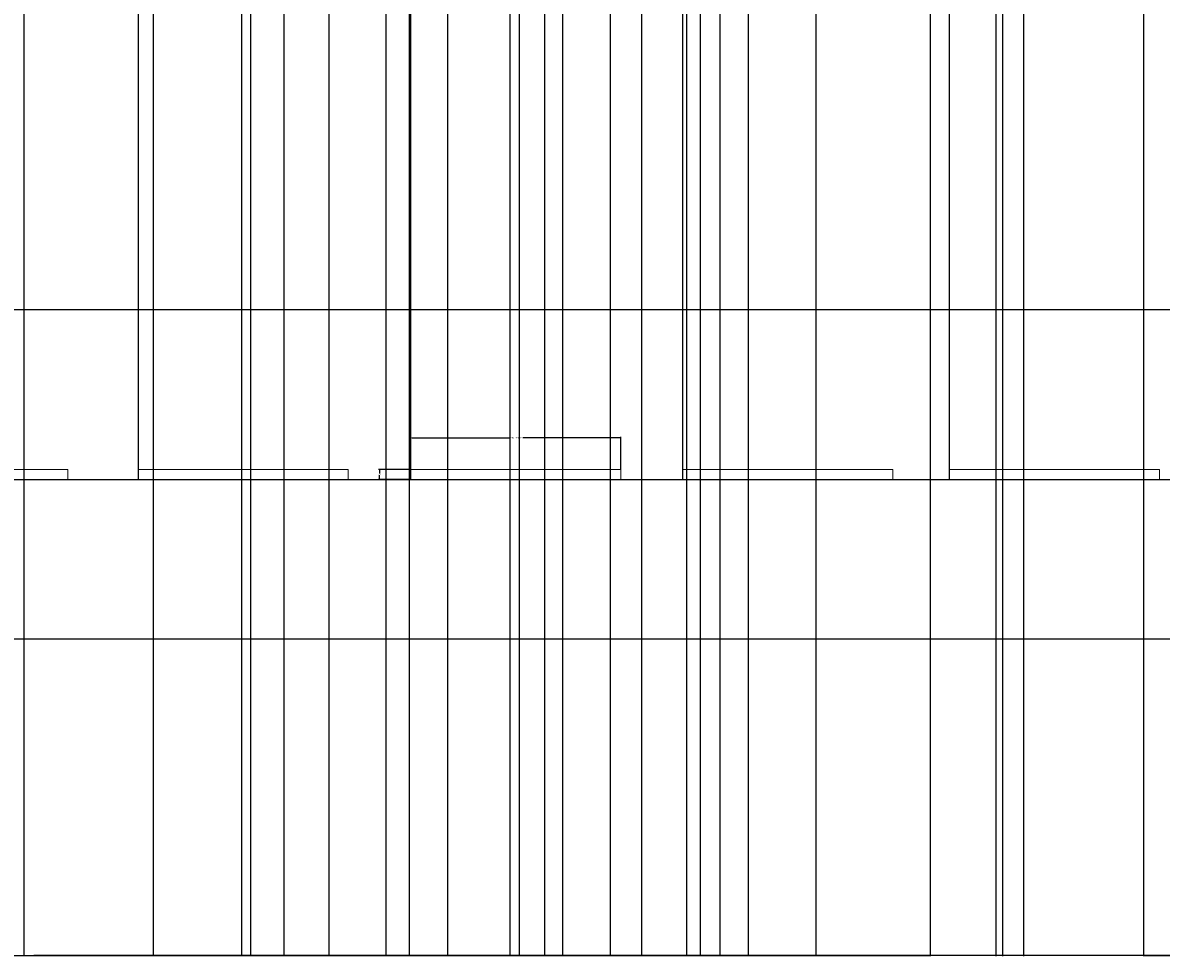
# Model space of a CAD drawing. Units: inches. Extents: x 818 to 1898, y 976 to 2364.
# Tile 14 of 96: x 1207 to 1434, y 976 to 1162. Entities that reach past the tile are written whole.
import ezdxf

# ---------------------------------------------------------------- set-up
doc = ezdxf.new("R2010")
doc.units = ezdxf.units.IN
doc.header["$LTSCALE"] = 5
doc.header["$MEASUREMENT"] = 0
for name, color, linetype, lineweight in [('A-ANNO-DIMS', 2, 'Continuous', 18), ('C-ROAD', 8, 'Continuous', 25), ('C-ROAD-MRKG', 7, 'Continuous', 13)]:
    doc.layers.add(name, color=color, linetype=linetype, lineweight=lineweight)
doc.styles.get("Standard").update_dxf_attribs({"font": 'arial.ttf'})
doc.dimstyles.get("Standard").update_dxf_attribs({"dimtxt": 0.18, "dimasz": 0.18, "dimexe": 0.18, "dimexo": 0.0625, "dimgap": 0.09, "dimtad": 0, "dimtih": 1, "dimtoh": 1, "dimdec": 4, "dimzin": 0, "dimdsep": 46, "dimtxsty": 'Standard', "dimcen": 0.09, "dimadec": 0, "dimazin": 0, "dimtfac": 1, "dimtdec": 4, "dimtofl": 0, "dimtmove": 0, "dimatfit": 3, "dimfxl": 1, "dimtolj": 1, "dimtzin": 0, "dimarcsym": 0})

# ---------------------------------------------------------------- blocks, each defined once
blk = doc.blocks.new('LANE-STRIPE')
at = {"ltscale": 5}
for p, q in [((0, 2), (42, 2)), ((0, 2), (0, 0)), ((0, 0), (42, 0)), ((42, 2), (42, 0))]:
    blk.add_line(p, q, dxfattribs=at)
blk = doc.blocks.new('*D32')
at = {"layer": 'A-ANNO-DIMS', "color": 0, "lineweight": -2, "ltscale": 5, "transparency": 16777216}
for p, q in [((1284.17, 1073.12), (1284.17, 1079.54)), ((1326.17, 1073.12), (1326.17, 1079.54)), ((1284.35, 1079.36), (1303.79, 1079.36)), ((1325.99, 1079.36), (1306.55, 1079.36))]:
    blk.add_line(p, q, dxfattribs=at)
at = {"layer": 'A-ANNO-DIMS', "color": 0, "ltscale": 5, "transparency": 16777216}
for points in [[(1284.35, 1079.39), (1284.35, 1079.33), (1284.17, 1079.36)], [(1325.99, 1079.39), (1325.99, 1079.33), (1326.17, 1079.36)]]:
    blk.add_solid(points, dxfattribs=at)
at = {"layer": 'Defpoints', "color": 0, "ltscale": 5, "transparency": 16777216}
for p in [(1284.17, 1079.36), (1284.17, 1073.06), (1326.17, 1073.06)]:
    blk.add_point(p, dxfattribs=at)
at = {"layer": 'A-ANNO-DIMS', "color": 0, "ltscale": 5, "transparency": 16777216, "insert": (1305.17, 1079.36), "char_height": 0.18, "attachment_point": 5}
blk.add_mtext('\\A1;LANE STRIPE 42 TYP.', dxfattribs=at)
blk = doc.blocks.new('*D33')
at = {"layer": 'A-ANNO-DIMS', "color": 0, "lineweight": -2, "ltscale": 5, "transparency": 16777216}
for p, q in [((1284.11, 1073.06), (1277.69, 1073.06)), ((1277.87, 1072.88), (1277.87, 1072.24)), ((1284.11, 1071.06), (1277.69, 1071.06)), ((1277.87, 1071.24), (1277.87, 1071.87))]:
    blk.add_line(p, q, dxfattribs=at)
at = {"layer": 'A-ANNO-DIMS', "color": 0, "ltscale": 5, "transparency": 16777216}
for points in [[(1277.84, 1072.88), (1277.9, 1072.88), (1277.87, 1073.06)], [(1277.84, 1071.24), (1277.9, 1071.24), (1277.87, 1071.06)]]:
    blk.add_solid(points, dxfattribs=at)
at = {"layer": 'Defpoints', "color": 0, "ltscale": 5, "transparency": 16777216}
for p in [(1284.17, 1073.06), (1277.87, 1071.06), (1284.17, 1071.06)]:
    blk.add_point(p, dxfattribs=at)
at = {"layer": 'A-ANNO-DIMS', "color": 0, "ltscale": 5, "transparency": 16777216, "insert": (1277.87, 1072.06), "char_height": 0.18, "attachment_point": 5}
blk.add_mtext('\\A1;2 TYP.', dxfattribs=at)
blk = doc.blocks.new('*D56')
at = {"layer": 'A-ANNO-DIMS', "color": 0, "lineweight": -2, "ltscale": 5, "transparency": 16777216}
for p, q in [((885.95, 1167.31), (885.95, 975.66)), ((1828.91, 1167.31), (1828.91, 975.66)), ((886.13, 975.84), (1357.14, 975.84)), ((1828.73, 975.84), (1357.72, 975.84))]:
    blk.add_line(p, q, dxfattribs=at)
at = {"layer": 'A-ANNO-DIMS', "color": 0, "ltscale": 5, "transparency": 16777216}
for points in [[(886.13, 975.87), (886.13, 975.81), (885.95, 975.84)], [(1828.73, 975.87), (1828.73, 975.81), (1828.91, 975.84)]]:
    blk.add_solid(points, dxfattribs=at)
at = {"layer": 'Defpoints', "color": 0, "ltscale": 5, "transparency": 16777216}
for p in [(885.95, 1167.37), (1828.91, 1167.37), (1828.91, 975.84)]:
    blk.add_point(p, dxfattribs=at)
at = {"layer": 'A-ANNO-DIMS', "color": 0, "ltscale": 5, "transparency": 16777216, "insert": (1357.43, 975.84), "char_height": 0.18, "attachment_point": 5}
blk.add_mtext('\\A1;943', dxfattribs=at)
blk = doc.blocks.new('*D58')
at = {"layer": 'A-ANNO-DIMS', "color": 0, "lineweight": -2, "ltscale": 5, "transparency": 16777216}
for p, q in [((881.51, 1159.31), (881.51, 975.66)), ((1834.44, 1145.13), (1834.44, 975.66)), ((881.69, 975.84), (1357.68, 975.84)), ((1834.26, 975.84), (1358.26, 975.84))]:
    blk.add_line(p, q, dxfattribs=at)
at = {"layer": 'A-ANNO-DIMS', "color": 0, "ltscale": 5, "transparency": 16777216}
for points in [[(881.69, 975.87), (881.69, 975.81), (881.51, 975.84)], [(1834.26, 975.87), (1834.26, 975.81), (1834.44, 975.84)]]:
    blk.add_solid(points, dxfattribs=at)
at = {"layer": 'Defpoints', "color": 0, "ltscale": 5, "transparency": 16777216}
for p in [(881.51, 1159.38), (1834.44, 1145.19), (1834.44, 975.84)]:
    blk.add_point(p, dxfattribs=at)
at = {"layer": 'A-ANNO-DIMS', "color": 0, "ltscale": 5, "transparency": 16777216, "insert": (1357.97, 975.84), "char_height": 0.18, "attachment_point": 5}
blk.add_mtext('\\A1;953', dxfattribs=at)
blk = doc.blocks.new('*D59')
at = {"layer": 'A-ANNO-DIMS', "color": 0, "lineweight": -2, "ltscale": 5, "transparency": 16777216}
for p, q in [((1251.64, 2300.39), (818.03, 2300.39)), ((818.21, 2300.21), (818.21, 1669.95)), ((818.21, 1039.32), (818.21, 1669.59)), ((896.05, 1039.14), (818.03, 1039.14))]:
    blk.add_line(p, q, dxfattribs=at)
at = {"layer": 'A-ANNO-DIMS', "color": 0, "ltscale": 5, "transparency": 16777216}
for points in [[(818.18, 2300.21), (818.24, 2300.21), (818.21, 2300.39)], [(818.18, 1039.32), (818.24, 1039.32), (818.21, 1039.14)]]:
    blk.add_solid(points, dxfattribs=at)
at = {"layer": 'Defpoints', "color": 0, "ltscale": 5, "transparency": 16777216}
for p in [(818.21, 2300.39), (1251.71, 2300.39), (896.11, 1039.14)]:
    blk.add_point(p, dxfattribs=at)
at = {"layer": 'A-ANNO-DIMS', "color": 0, "ltscale": 5, "transparency": 16777216, "insert": (818.21, 1669.77), "char_height": 0.18, "attachment_point": 5}
blk.add_mtext('\\A1;1261.2', dxfattribs=at)
blk = doc.blocks.new('*D62')
at = {"layer": 'A-ANNO-DIMS', "color": 0, "lineweight": -2, "ltscale": 5, "transparency": 16777216}
for p, q in [((1116.19, 1235.9), (1116.19, 975.66)), ((1406.73, 1235.9), (1406.73, 975.66)), ((1116.37, 975.84), (1260.99, 975.84)), ((1406.55, 975.84), (1261.92, 975.84))]:
    blk.add_line(p, q, dxfattribs=at)
at = {"layer": 'A-ANNO-DIMS', "color": 0, "ltscale": 5, "transparency": 16777216}
for points in [[(1116.37, 975.87), (1116.37, 975.81), (1116.19, 975.84)], [(1406.55, 975.87), (1406.55, 975.81), (1406.73, 975.84)]]:
    blk.add_solid(points, dxfattribs=at)
at = {"layer": 'Defpoints', "color": 0, "ltscale": 5, "transparency": 16777216}
for p in [(1116.19, 1235.96), (1406.73, 1235.96), (1406.73, 975.84)]:
    blk.add_point(p, dxfattribs=at)
at = {"layer": 'A-ANNO-DIMS', "color": 0, "ltscale": 5, "transparency": 16777216, "insert": (1261.46, 975.84), "char_height": 0.18, "attachment_point": 5}
blk.add_mtext('\\A1;290.54', dxfattribs=at)
blk = doc.blocks.new('*D65')
at = {"layer": 'A-ANNO-DIMS', "color": 0, "lineweight": -2, "ltscale": 5, "transparency": 16777216}
for p, q in [((1430.73, 1346.02), (1430.73, 975.66)), ((1714.73, 1346.02), (1714.73, 975.66)), ((1430.91, 975.84), (1572.44, 975.84)), ((1714.55, 975.84), (1573.02, 975.84))]:
    blk.add_line(p, q, dxfattribs=at)
at = {"layer": 'A-ANNO-DIMS', "color": 0, "ltscale": 5, "transparency": 16777216}
for points in [[(1430.91, 975.87), (1430.91, 975.81), (1430.73, 975.84)], [(1714.55, 975.87), (1714.55, 975.81), (1714.73, 975.84)]]:
    blk.add_solid(points, dxfattribs=at)
at = {"layer": 'Defpoints', "color": 0, "ltscale": 5, "transparency": 16777216}
for p in [(1430.73, 1346.08), (1714.73, 1346.08), (1714.73, 975.84)]:
    blk.add_point(p, dxfattribs=at)
at = {"layer": 'A-ANNO-DIMS', "color": 0, "ltscale": 5, "transparency": 16777216, "insert": (1572.73, 975.84), "char_height": 0.18, "attachment_point": 5}
blk.add_mtext('\\A1;284', dxfattribs=at)
blk = doc.blocks.new('*D89')
at = {"layer": 'A-ANNO-DIMS', "color": 0, "lineweight": -2, "ltscale": 5, "transparency": 16777216}
for p, q in [((905.01, 1071.06), (1897.92, 1071.06)), ((1897.74, 1070.88), (1897.74, 1055.28)), ((1897.74, 1039.32), (1897.74, 1054.92)), ((896.18, 1039.14), (1897.92, 1039.14))]:
    blk.add_line(p, q, dxfattribs=at)
at = {"layer": 'A-ANNO-DIMS', "color": 0, "ltscale": 5, "transparency": 16777216}
for points in [[(1897.71, 1070.88), (1897.77, 1070.88), (1897.74, 1071.06)], [(1897.71, 1039.32), (1897.77, 1039.32), (1897.74, 1039.14)]]:
    blk.add_solid(points, dxfattribs=at)
at = {"layer": 'Defpoints', "color": 0, "ltscale": 5, "transparency": 16777216}
for p in [(904.95, 1071.06), (1897.74, 1071.06), (896.11, 1039.14)]:
    blk.add_point(p, dxfattribs=at)
at = {"layer": 'A-ANNO-DIMS', "color": 0, "ltscale": 5, "transparency": 16777216, "insert": (1897.74, 1055.1), "char_height": 0.18, "attachment_point": 5}
blk.add_mtext('\\A1;31.91', dxfattribs=at)
blk = doc.blocks.new('*D95')
at = {"layer": 'A-ANNO-DIMS', "color": 0, "lineweight": -2, "ltscale": 5, "transparency": 16777216}
for p, q in [((1173.54, 1071.12), (1173.54, 2363.87)), ((1229.65, 1071.12), (1229.65, 2363.87)), ((1173.72, 2363.69), (1201.29, 2363.69)), ((1229.47, 2363.69), (1201.9, 2363.69))]:
    blk.add_line(p, q, dxfattribs=at)
at = {"layer": 'A-ANNO-DIMS', "color": 0, "ltscale": 5, "transparency": 16777216}
for points in [[(1173.72, 2363.72), (1173.72, 2363.66), (1173.54, 2363.69)], [(1229.47, 2363.72), (1229.47, 2363.66), (1229.65, 2363.69)]]:
    blk.add_solid(points, dxfattribs=at)
at = {"layer": 'Defpoints', "color": 0, "ltscale": 5, "transparency": 16777216}
for p in [(1229.65, 2363.69), (1173.54, 1071.06), (1229.65, 1071.06)]:
    blk.add_point(p, dxfattribs=at)
at = {"layer": 'A-ANNO-DIMS', "color": 0, "ltscale": 5, "transparency": 16777216, "insert": (1201.59, 2363.69), "char_height": 0.18, "attachment_point": 5}
blk.add_mtext('\\A1;56.1', dxfattribs=at)
blk = doc.blocks.new('*D96')
at = {"layer": 'A-ANNO-DIMS', "color": 0, "lineweight": -2, "ltscale": 5, "transparency": 16777216}
for p, q in [((1229.65, 1071.12), (1229.65, 2363.87)), ((1284.17, 1071.12), (1284.17, 2363.87)), ((1229.83, 2363.69), (1256.52, 2363.69)), ((1283.99, 2363.69), (1257.3, 2363.69))]:
    blk.add_line(p, q, dxfattribs=at)
at = {"layer": 'A-ANNO-DIMS', "color": 0, "ltscale": 5, "transparency": 16777216}
for points in [[(1229.83, 2363.72), (1229.83, 2363.66), (1229.65, 2363.69)], [(1283.99, 2363.72), (1283.99, 2363.66), (1284.17, 2363.69)]]:
    blk.add_solid(points, dxfattribs=at)
at = {"layer": 'Defpoints', "color": 0, "ltscale": 5, "transparency": 16777216}
for p in [(1284.17, 2363.69), (1229.65, 1071.06), (1284.17, 1071.06)]:
    blk.add_point(p, dxfattribs=at)
at = {"layer": 'A-ANNO-DIMS', "color": 0, "ltscale": 5, "transparency": 16777216, "insert": (1256.91, 2363.69), "char_height": 0.18, "attachment_point": 5}
blk.add_mtext('\\A1;54.52', dxfattribs=at)
blk = doc.blocks.new('*D97')
at = {"layer": 'A-ANNO-DIMS', "color": 0, "lineweight": -2, "ltscale": 5, "transparency": 16777216}
for p, q in [((1284.17, 1071.12), (1284.17, 2363.87)), ((1338.54, 1071.12), (1338.54, 2363.87)), ((1284.35, 2363.69), (1310.96, 2363.69)), ((1338.36, 2363.69), (1311.75, 2363.69))]:
    blk.add_line(p, q, dxfattribs=at)
at = {"layer": 'A-ANNO-DIMS', "color": 0, "ltscale": 5, "transparency": 16777216}
for points in [[(1284.35, 2363.72), (1284.35, 2363.66), (1284.17, 2363.69)], [(1338.36, 2363.72), (1338.36, 2363.66), (1338.54, 2363.69)]]:
    blk.add_solid(points, dxfattribs=at)
at = {"layer": 'Defpoints', "color": 0, "ltscale": 5, "transparency": 16777216}
for p in [(1338.54, 2363.69), (1284.17, 1071.06), (1338.54, 1071.06)]:
    blk.add_point(p, dxfattribs=at)
at = {"layer": 'A-ANNO-DIMS', "color": 0, "ltscale": 5, "transparency": 16777216, "insert": (1311.36, 2363.69), "char_height": 0.18, "attachment_point": 5}
blk.add_mtext('\\A1;54.37', dxfattribs=at)
blk = doc.blocks.new('*D98')
at = {"layer": 'A-ANNO-DIMS', "color": 0, "lineweight": -2, "ltscale": 5, "transparency": 16777216}
for p, q in [((1338.54, 1071.12), (1338.54, 2363.87)), ((1391.88, 1071.12), (1391.88, 2363.87)), ((1338.72, 2363.69), (1364.81, 2363.69)), ((1391.7, 2363.69), (1365.6, 2363.69))]:
    blk.add_line(p, q, dxfattribs=at)
at = {"layer": 'A-ANNO-DIMS', "color": 0, "ltscale": 5, "transparency": 16777216}
for points in [[(1338.72, 2363.72), (1338.72, 2363.66), (1338.54, 2363.69)], [(1391.7, 2363.72), (1391.7, 2363.66), (1391.88, 2363.69)]]:
    blk.add_solid(points, dxfattribs=at)
at = {"layer": 'Defpoints', "color": 0, "ltscale": 5, "transparency": 16777216}
for p in [(1391.88, 2363.69), (1338.54, 1071.06), (1391.88, 1071.06)]:
    blk.add_point(p, dxfattribs=at)
at = {"layer": 'A-ANNO-DIMS', "color": 0, "ltscale": 5, "transparency": 16777216, "insert": (1365.21, 2363.69), "char_height": 0.18, "attachment_point": 5}
blk.add_mtext('\\A1;53.33', dxfattribs=at)
blk = doc.blocks.new('*D99')
at = {"layer": 'A-ANNO-DIMS', "color": 0, "lineweight": -2, "ltscale": 5, "transparency": 16777216}
for p, q in [((1391.88, 1071.12), (1391.88, 2363.87)), ((1449.82, 1071.12), (1449.82, 2363.87)), ((1392.06, 2363.69), (1420.45, 2363.69)), ((1449.64, 2363.69), (1421.24, 2363.69))]:
    blk.add_line(p, q, dxfattribs=at)
at = {"layer": 'A-ANNO-DIMS', "color": 0, "ltscale": 5, "transparency": 16777216}
for points in [[(1392.06, 2363.72), (1392.06, 2363.66), (1391.88, 2363.69)], [(1449.64, 2363.72), (1449.64, 2363.66), (1449.82, 2363.69)]]:
    blk.add_solid(points, dxfattribs=at)
at = {"layer": 'Defpoints', "color": 0, "ltscale": 5, "transparency": 16777216}
for p in [(1449.82, 2363.69), (1391.88, 1071.06), (1449.82, 1071.06)]:
    blk.add_point(p, dxfattribs=at)
at = {"layer": 'A-ANNO-DIMS', "color": 0, "ltscale": 5, "transparency": 16777216, "insert": (1420.85, 2363.69), "char_height": 0.18, "attachment_point": 5}
blk.add_mtext('\\A1;57.94', dxfattribs=at)
blk = doc.blocks.new('*D106')
at = {"layer": 'A-ANNO-DIMS', "color": 0, "lineweight": -2, "ltscale": 5, "transparency": 16777216}
for p, q in [((1164.56, 1248.4), (1164.56, 975.66)), ((1252.11, 1248.4), (1252.11, 975.66)), ((1164.74, 975.84), (1207.94, 975.84)), ((1251.93, 975.84), (1208.73, 975.84))]:
    blk.add_line(p, q, dxfattribs=at)
at = {"layer": 'A-ANNO-DIMS', "color": 0, "ltscale": 5, "transparency": 16777216}
for points in [[(1164.74, 975.87), (1164.74, 975.81), (1164.56, 975.84)], [(1251.93, 975.87), (1251.93, 975.81), (1252.11, 975.84)]]:
    blk.add_solid(points, dxfattribs=at)
at = {"layer": 'Defpoints', "color": 0, "ltscale": 5, "transparency": 16777216}
for p in [(1164.56, 1248.46), (1252.11, 1248.46), (1252.11, 975.84)]:
    blk.add_point(p, dxfattribs=at)
at = {"layer": 'A-ANNO-DIMS', "color": 0, "ltscale": 5, "transparency": 16777216, "insert": (1208.33, 975.84), "char_height": 0.18, "attachment_point": 5}
blk.add_mtext('\\A1;87.55', dxfattribs=at)
blk = doc.blocks.new('*D107')
at = {"layer": 'A-ANNO-DIMS', "color": 0, "lineweight": -2, "ltscale": 5, "transparency": 16777216}
for p, q in [((1339.32, 1250.56), (1339.32, 975.66)), ((1252.11, 1248.4), (1252.11, 975.66)), ((1252.29, 975.84), (1295.39, 975.84)), ((1339.14, 975.84), (1296.04, 975.84))]:
    blk.add_line(p, q, dxfattribs=at)
at = {"layer": 'A-ANNO-DIMS', "color": 0, "ltscale": 5, "transparency": 16777216}
for points in [[(1252.29, 975.87), (1252.29, 975.81), (1252.11, 975.84)], [(1339.14, 975.87), (1339.14, 975.81), (1339.32, 975.84)]]:
    blk.add_solid(points, dxfattribs=at)
at = {"layer": 'Defpoints', "color": 0, "ltscale": 5, "transparency": 16777216}
for p in [(1339.32, 1250.62), (1252.11, 1248.46), (1339.32, 975.84)]:
    blk.add_point(p, dxfattribs=at)
at = {"layer": 'A-ANNO-DIMS', "color": 0, "ltscale": 5, "transparency": 16777216, "insert": (1295.71, 975.84), "char_height": 0.18, "attachment_point": 5}
blk.add_mtext('\\A1;87.2', dxfattribs=at)
blk = doc.blocks.new('*D145')
at = {"layer": 'A-ANNO-DIMS', "color": 0, "lineweight": -2, "ltscale": 5, "transparency": 16777216}
for p, q in [((1197.39, 2122.31), (1197.39, 975.66)), ((1232.61, 2122.31), (1232.61, 975.66)), ((1197.57, 975.84), (1214.61, 975.84)), ((1232.43, 975.84), (1215.39, 975.84))]:
    blk.add_line(p, q, dxfattribs=at)
at = {"layer": 'A-ANNO-DIMS', "color": 0, "ltscale": 5, "transparency": 16777216}
for points in [[(1197.57, 975.87), (1197.57, 975.81), (1197.39, 975.84)], [(1232.43, 975.87), (1232.43, 975.81), (1232.61, 975.84)]]:
    blk.add_solid(points, dxfattribs=at)
at = {"layer": 'Defpoints', "color": 0, "ltscale": 5, "transparency": 16777216}
for p in [(1197.39, 2122.38), (1232.61, 2122.38), (1232.61, 975.84)]:
    blk.add_point(p, dxfattribs=at)
at = {"layer": 'A-ANNO-DIMS', "color": 0, "ltscale": 5, "transparency": 16777216, "insert": (1215, 975.84), "char_height": 0.18, "attachment_point": 5}
blk.add_mtext('\\A1;35.22', dxfattribs=at)
blk = doc.blocks.new('*D159')
at = {"layer": 'A-ANNO-DIMS', "color": 0, "lineweight": -2, "ltscale": 5, "transparency": 16777216}
for p, q in [((1206.73, 1687.02), (1206.73, 975.66)), ((1463.73, 1687.02), (1463.73, 975.66)), ((1206.91, 975.84), (1334.93, 975.84)), ((1463.55, 975.84), (1335.52, 975.84))]:
    blk.add_line(p, q, dxfattribs=at)
at = {"layer": 'A-ANNO-DIMS', "color": 0, "ltscale": 5, "transparency": 16777216}
for points in [[(1206.91, 975.87), (1206.91, 975.81), (1206.73, 975.84)], [(1463.55, 975.87), (1463.55, 975.81), (1463.73, 975.84)]]:
    blk.add_solid(points, dxfattribs=at)
at = {"layer": 'Defpoints', "color": 0, "ltscale": 5, "transparency": 16777216}
for p in [(1206.73, 1687.08), (1463.73, 1687.08), (1463.73, 975.84)]:
    blk.add_point(p, dxfattribs=at)
at = {"layer": 'A-ANNO-DIMS', "color": 0, "ltscale": 5, "transparency": 16777216, "insert": (1335.23, 975.84), "char_height": 0.18, "attachment_point": 5}
blk.add_mtext('\\A1;257', dxfattribs=at)
blk = doc.blocks.new('*D163')
at = {"layer": 'A-ANNO-DIMS', "color": 0, "lineweight": -2, "ltscale": 5, "transparency": 16777216}
for p, q in [((1365.15, 1501.02), (1365.15, 975.66)), ((1401.15, 1501.02), (1401.15, 975.66)), ((1365.33, 975.84), (1382.93, 975.84)), ((1400.97, 975.84), (1383.37, 975.84))]:
    blk.add_line(p, q, dxfattribs=at)
at = {"layer": 'A-ANNO-DIMS', "color": 0, "ltscale": 5, "transparency": 16777216}
for points in [[(1365.33, 975.87), (1365.33, 975.81), (1365.15, 975.84)], [(1400.97, 975.87), (1400.97, 975.81), (1401.15, 975.84)]]:
    blk.add_solid(points, dxfattribs=at)
at = {"layer": 'Defpoints', "color": 0, "ltscale": 5, "transparency": 16777216}
for p in [(1365.15, 1501.08), (1401.15, 1501.08), (1401.15, 975.84)]:
    blk.add_point(p, dxfattribs=at)
at = {"layer": 'A-ANNO-DIMS', "color": 0, "ltscale": 5, "transparency": 16777216, "insert": (1383.15, 975.84), "char_height": 0.18, "attachment_point": 5}
blk.add_mtext('\\A1;36', dxfattribs=at)
blk = doc.blocks.new('*D164')
at = {"layer": 'A-ANNO-DIMS', "color": 0, "lineweight": -2, "ltscale": 5, "transparency": 16777216}
for p, q in [((1206.73, 1501.02), (1206.73, 975.66)), ((1283.82, 1501.02), (1283.82, 975.66)), ((1206.91, 975.84), (1244.97, 975.84)), ((1283.64, 975.84), (1245.58, 975.84))]:
    blk.add_line(p, q, dxfattribs=at)
at = {"layer": 'A-ANNO-DIMS', "color": 0, "ltscale": 5, "transparency": 16777216}
for points in [[(1206.91, 975.87), (1206.91, 975.81), (1206.73, 975.84)], [(1283.64, 975.87), (1283.64, 975.81), (1283.82, 975.84)]]:
    blk.add_solid(points, dxfattribs=at)
at = {"layer": 'Defpoints', "color": 0, "ltscale": 5, "transparency": 16777216}
for p in [(1206.73, 1501.08), (1283.82, 1501.08), (1283.82, 975.84)]:
    blk.add_point(p, dxfattribs=at)
at = {"layer": 'A-ANNO-DIMS', "color": 0, "ltscale": 5, "transparency": 16777216, "insert": (1245.27, 975.84), "char_height": 0.18, "attachment_point": 5}
blk.add_mtext('\\A1;77.1', dxfattribs=at)
blk = doc.blocks.new('*D167')
at = {"layer": 'A-ANNO-DIMS', "color": 0, "lineweight": -2, "ltscale": 5, "transparency": 16777216}
for p, q in [((1345.97, 1486.18), (1345.97, 975.66)), ((1430.73, 1486.18), (1430.73, 975.66)), ((1346.15, 975.84), (1387.95, 975.84)), ((1430.55, 975.84), (1388.74, 975.84))]:
    blk.add_line(p, q, dxfattribs=at)
at = {"layer": 'A-ANNO-DIMS', "color": 0, "ltscale": 5, "transparency": 16777216}
for points in [[(1346.15, 975.87), (1346.15, 975.81), (1345.97, 975.84)], [(1430.55, 975.87), (1430.55, 975.81), (1430.73, 975.84)]]:
    blk.add_solid(points, dxfattribs=at)
at = {"layer": 'Defpoints', "color": 0, "ltscale": 5, "transparency": 16777216}
for p in [(1345.97, 1486.24), (1430.73, 1486.24), (1430.73, 975.84)]:
    blk.add_point(p, dxfattribs=at)
at = {"layer": 'A-ANNO-DIMS', "color": 0, "ltscale": 5, "transparency": 16777216, "insert": (1388.35, 975.84), "char_height": 0.18, "attachment_point": 5}
blk.add_mtext('\\A1;84.76', dxfattribs=at)
blk = doc.blocks.new('*D189')
at = {"layer": 'A-ANNO-DIMS', "color": 0, "lineweight": -2, "ltscale": 5, "transparency": 16777216}
for p, q in [((1430.73, 1346.02), (1430.73, 975.66)), ((1490.92, 1346.02), (1490.92, 975.66)), ((1430.91, 975.84), (1460.43, 975.84)), ((1490.74, 975.84), (1461.22, 975.84))]:
    blk.add_line(p, q, dxfattribs=at)
at = {"layer": 'A-ANNO-DIMS', "color": 0, "ltscale": 5, "transparency": 16777216}
for points in [[(1430.91, 975.87), (1430.91, 975.81), (1430.73, 975.84)], [(1490.74, 975.87), (1490.74, 975.81), (1490.92, 975.84)]]:
    blk.add_solid(points, dxfattribs=at)
at = {"layer": 'Defpoints', "color": 0, "ltscale": 5, "transparency": 16777216}
for p in [(1430.73, 1346.08), (1490.92, 1346.08), (1490.92, 975.84)]:
    blk.add_point(p, dxfattribs=at)
at = {"layer": 'A-ANNO-DIMS', "color": 0, "ltscale": 5, "transparency": 16777216, "insert": (1460.82, 975.84), "char_height": 0.18, "attachment_point": 5}
blk.add_mtext('\\A1;60.19', dxfattribs=at)
blk = doc.blocks.new('*D198')
at = {"layer": 'A-ANNO-DIMS', "color": 0, "lineweight": -2, "ltscale": 5, "transparency": 16777216}
for p, q in [((1741.84, 1545.02), (1741.84, 975.66)), ((1430.73, 1346.02), (1430.73, 975.66)), ((1430.91, 975.84), (1585.91, 975.84)), ((1741.66, 975.84), (1586.66, 975.84))]:
    blk.add_line(p, q, dxfattribs=at)
at = {"layer": 'A-ANNO-DIMS', "color": 0, "ltscale": 5, "transparency": 16777216}
for points in [[(1430.91, 975.87), (1430.91, 975.81), (1430.73, 975.84)], [(1741.66, 975.87), (1741.66, 975.81), (1741.84, 975.84)]]:
    blk.add_solid(points, dxfattribs=at)
at = {"layer": 'Defpoints', "color": 0, "ltscale": 5, "transparency": 16777216}
for p in [(1741.84, 1545.08), (1430.73, 1346.08), (1741.84, 975.84)]:
    blk.add_point(p, dxfattribs=at)
at = {"layer": 'A-ANNO-DIMS', "color": 0, "ltscale": 5, "transparency": 16777216, "insert": (1586.28, 975.84), "char_height": 0.18, "attachment_point": 5}
blk.add_mtext('\\A1;311.1', dxfattribs=at)
blk = doc.blocks.new('*D231')
at = {"layer": 'A-ANNO-DIMS', "color": 0, "lineweight": -2, "ltscale": 5, "transparency": 16777216}
for p, q in [((1303.93, 1952.98), (1303.93, 975.66)), ((1402.52, 1952.98), (1402.52, 975.66)), ((1304.11, 975.84), (1352.83, 975.84)), ((1402.34, 975.84), (1353.62, 975.84))]:
    blk.add_line(p, q, dxfattribs=at)
at = {"layer": 'A-ANNO-DIMS', "color": 0, "ltscale": 5, "transparency": 16777216}
for points in [[(1304.11, 975.87), (1304.11, 975.81), (1303.93, 975.84)], [(1402.34, 975.87), (1402.34, 975.81), (1402.52, 975.84)]]:
    blk.add_solid(points, dxfattribs=at)
at = {"layer": 'Defpoints', "color": 0, "ltscale": 5, "transparency": 16777216}
for p in [(1303.93, 1953.04), (1402.52, 1953.04), (1402.52, 975.84)]:
    blk.add_point(p, dxfattribs=at)
at = {"layer": 'A-ANNO-DIMS', "color": 0, "ltscale": 5, "transparency": 16777216, "insert": (1353.22, 975.84), "char_height": 0.18, "attachment_point": 5}
blk.add_mtext('\\A1;98.59', dxfattribs=at)
blk = doc.blocks.new('*D233')
at = {"layer": 'A-ANNO-DIMS', "color": 0, "lineweight": -2, "ltscale": 5, "transparency": 16777216}
for p, q in [((1267.73, 2044.02), (1267.73, 975.66)), ((1303.93, 2008.33), (1303.93, 975.66)), ((1267.91, 975.84), (1285.36, 975.84)), ((1303.75, 975.84), (1286.29, 975.84))]:
    blk.add_line(p, q, dxfattribs=at)
at = {"layer": 'A-ANNO-DIMS', "color": 0, "ltscale": 5, "transparency": 16777216}
for points in [[(1267.91, 975.87), (1267.91, 975.81), (1267.73, 975.84)], [(1303.75, 975.87), (1303.75, 975.81), (1303.93, 975.84)]]:
    blk.add_solid(points, dxfattribs=at)
at = {"layer": 'Defpoints', "color": 0, "ltscale": 5, "transparency": 16777216}
for p in [(1267.73, 2044.08), (1303.93, 2008.39), (1303.93, 975.84)]:
    blk.add_point(p, dxfattribs=at)
at = {"layer": 'A-ANNO-DIMS', "color": 0, "ltscale": 5, "transparency": 16777216, "insert": (1285.83, 975.84), "char_height": 0.18, "attachment_point": 5}
blk.add_mtext('\\A1;36.206', dxfattribs=at)
blk = doc.blocks.new('*D236')
at = {"layer": 'A-ANNO-DIMS', "color": 0, "lineweight": -2, "ltscale": 5, "transparency": 16777216}
for p, q in [((1310.91, 2026.14), (1310.91, 975.66)), ((1342.04, 2026.14), (1342.04, 975.66)), ((1311.09, 975.84), (1326.08, 975.84)), ((1341.86, 975.84), (1326.87, 975.84))]:
    blk.add_line(p, q, dxfattribs=at)
at = {"layer": 'A-ANNO-DIMS', "color": 0, "ltscale": 5, "transparency": 16777216}
for points in [[(1311.09, 975.87), (1311.09, 975.81), (1310.91, 975.84)], [(1341.86, 975.87), (1341.86, 975.81), (1342.04, 975.84)]]:
    blk.add_solid(points, dxfattribs=at)
at = {"layer": 'Defpoints', "color": 0, "ltscale": 5, "transparency": 16777216}
for p in [(1310.91, 2026.21), (1342.04, 2026.21), (1342.04, 975.84)]:
    blk.add_point(p, dxfattribs=at)
at = {"layer": 'A-ANNO-DIMS', "color": 0, "ltscale": 5, "transparency": 16777216, "insert": (1326.48, 975.84), "char_height": 0.18, "attachment_point": 5}
blk.add_mtext('\\A1;31.14', dxfattribs=at)
blk = doc.blocks.new('*D245')
at = {"layer": 'A-ANNO-DIMS', "color": 0, "lineweight": -2, "ltscale": 5, "transparency": 16777216}
for p, q in [((1291.48, 1599.31), (1291.48, 975.66)), ((1314.49, 1599.31), (1314.49, 975.66)), ((1291.66, 975.84), (1302.61, 975.84)), ((1314.31, 975.84), (1303.36, 975.84))]:
    blk.add_line(p, q, dxfattribs=at)
at = {"layer": 'A-ANNO-DIMS', "color": 0, "ltscale": 5, "transparency": 16777216}
for points in [[(1291.66, 975.87), (1291.66, 975.81), (1291.48, 975.84)], [(1314.31, 975.87), (1314.31, 975.81), (1314.49, 975.84)]]:
    blk.add_solid(points, dxfattribs=at)
at = {"layer": 'Defpoints', "color": 0, "ltscale": 5, "transparency": 16777216}
for p in [(1291.48, 1599.37), (1314.49, 1599.37), (1314.49, 975.84)]:
    blk.add_point(p, dxfattribs=at)
at = {"layer": 'A-ANNO-DIMS', "color": 0, "ltscale": 5, "transparency": 16777216, "insert": (1302.98, 975.84), "char_height": 0.18, "attachment_point": 5}
blk.add_mtext('\\A1;23.01', dxfattribs=at)
blk = doc.blocks.new('*D251')
at = {"layer": 'A-ANNO-DIMS', "color": 0, "lineweight": -2, "ltscale": 5, "transparency": 16777216}
for p, q in [((1250.3, 1878.33), (1250.3, 975.66)), ((1258.73, 1878.33), (1258.73, 975.66)), ((1250.48, 975.84), (1254.12, 975.84)), ((1258.55, 975.84), (1254.91, 975.84))]:
    blk.add_line(p, q, dxfattribs=at)
at = {"layer": 'A-ANNO-DIMS', "color": 0, "ltscale": 5, "transparency": 16777216}
for points in [[(1250.48, 975.87), (1250.48, 975.81), (1250.3, 975.84)], [(1258.55, 975.87), (1258.55, 975.81), (1258.73, 975.84)]]:
    blk.add_solid(points, dxfattribs=at)
at = {"layer": 'Defpoints', "color": 0, "ltscale": 5, "transparency": 16777216}
for p in [(1250.3, 1878.39), (1258.73, 1878.39), (1258.73, 975.84)]:
    blk.add_point(p, dxfattribs=at)
at = {"layer": 'A-ANNO-DIMS', "color": 0, "ltscale": 5, "transparency": 16777216, "insert": (1254.51, 975.84), "char_height": 0.18, "attachment_point": 5}
blk.add_mtext('\\A1;8.422', dxfattribs=at)
blk = doc.blocks.new('*D252')
at = {"layer": 'A-ANNO-DIMS', "color": 0, "lineweight": -2, "ltscale": 5, "transparency": 16777216}
for p, q in [((1330.3, 2053.02), (1330.3, 975.66)), ((1388.03, 2053.02), (1388.03, 975.66)), ((1330.48, 975.84), (1358.77, 975.84)), ((1387.85, 975.84), (1359.56, 975.84))]:
    blk.add_line(p, q, dxfattribs=at)
at = {"layer": 'A-ANNO-DIMS', "color": 0, "ltscale": 5, "transparency": 16777216}
for points in [[(1330.48, 975.87), (1330.48, 975.81), (1330.3, 975.84)], [(1387.85, 975.87), (1387.85, 975.81), (1388.03, 975.84)]]:
    blk.add_solid(points, dxfattribs=at)
at = {"layer": 'Defpoints', "color": 0, "ltscale": 5, "transparency": 16777216}
for p in [(1330.3, 2053.08), (1388.03, 2053.08), (1388.03, 975.84)]:
    blk.add_point(p, dxfattribs=at)
at = {"layer": 'A-ANNO-DIMS', "color": 0, "ltscale": 5, "transparency": 16777216, "insert": (1359.17, 975.84), "char_height": 0.18, "attachment_point": 5}
blk.add_mtext('\\A1;57.73', dxfattribs=at)
blk = doc.blocks.new('*D254')
at = {"layer": 'A-ANNO-DIMS', "color": 0, "lineweight": -2, "ltscale": 5, "transparency": 16777216}
for p, q in [((1267.73, 2044.02), (1267.73, 975.66)), ((1330.3, 2044.02), (1330.3, 975.66)), ((1267.91, 975.84), (1298.62, 975.84)), ((1330.12, 975.84), (1299.41, 975.84))]:
    blk.add_line(p, q, dxfattribs=at)
at = {"layer": 'A-ANNO-DIMS', "color": 0, "ltscale": 5, "transparency": 16777216}
for points in [[(1267.91, 975.87), (1267.91, 975.81), (1267.73, 975.84)], [(1330.12, 975.87), (1330.12, 975.81), (1330.3, 975.84)]]:
    blk.add_solid(points, dxfattribs=at)
at = {"layer": 'Defpoints', "color": 0, "ltscale": 5, "transparency": 16777216}
for p in [(1267.73, 2044.08), (1330.3, 2044.08), (1330.3, 975.84)]:
    blk.add_point(p, dxfattribs=at)
at = {"layer": 'A-ANNO-DIMS', "color": 0, "ltscale": 5, "transparency": 16777216, "insert": (1299.02, 975.84), "char_height": 0.18, "attachment_point": 5}
blk.add_mtext('\\A1;62.58', dxfattribs=at)
blk = doc.blocks.new('*D278')
at = {"layer": 'A-ANNO-DIMS', "color": 0, "lineweight": -2, "ltscale": 5, "transparency": 16777216}
for p, q in [((1324.03, 1700.74), (1324.03, 975.66)), ((1267.73, 1696.02), (1267.73, 975.66)), ((1267.91, 975.84), (1295.5, 975.84)), ((1323.85, 975.84), (1296.26, 975.84))]:
    blk.add_line(p, q, dxfattribs=at)
at = {"layer": 'A-ANNO-DIMS', "color": 0, "ltscale": 5, "transparency": 16777216}
for points in [[(1267.91, 975.87), (1267.91, 975.81), (1267.73, 975.84)], [(1323.85, 975.87), (1323.85, 975.81), (1324.03, 975.84)]]:
    blk.add_solid(points, dxfattribs=at)
at = {"layer": 'Defpoints', "color": 0, "ltscale": 5, "transparency": 16777216}
for p in [(1324.03, 1700.81), (1267.73, 1696.08), (1324.03, 975.84)]:
    blk.add_point(p, dxfattribs=at)
at = {"layer": 'A-ANNO-DIMS', "color": 0, "ltscale": 5, "transparency": 16777216, "insert": (1295.88, 975.84), "char_height": 0.18, "attachment_point": 5}
blk.add_mtext('\\A1;56.31', dxfattribs=at)
blk = doc.blocks.new('*D279')
at = {"layer": 'A-ANNO-DIMS', "color": 0, "lineweight": -2, "ltscale": 5, "transparency": 16777216}
for p, q in [((1279.13, 1713.75), (1279.13, 975.66)), ((1267.73, 1696.02), (1267.73, 975.66)), ((1267.91, 975.84), (1273.11, 975.84)), ((1278.95, 975.84), (1273.74, 975.84))]:
    blk.add_line(p, q, dxfattribs=at)
at = {"layer": 'A-ANNO-DIMS', "color": 0, "ltscale": 5, "transparency": 16777216}
for points in [[(1267.91, 975.87), (1267.91, 975.81), (1267.73, 975.84)], [(1278.95, 975.87), (1278.95, 975.81), (1279.13, 975.84)]]:
    blk.add_solid(points, dxfattribs=at)
at = {"layer": 'Defpoints', "color": 0, "ltscale": 5, "transparency": 16777216}
for p in [(1279.13, 1713.82), (1267.73, 1696.08), (1267.73, 975.84)]:
    blk.add_point(p, dxfattribs=at)
at = {"layer": 'A-ANNO-DIMS', "color": 0, "ltscale": 5, "transparency": 16777216, "insert": (1273.43, 975.84), "char_height": 0.18, "attachment_point": 5}
blk.add_mtext('\\A1;11.4', dxfattribs=at)
blk = doc.blocks.new('*D283')
at = {"layer": 'A-ANNO-DIMS', "color": 0, "lineweight": -2, "ltscale": 5, "transparency": 16777216}
for p, q in [((1351.6, 1761.39), (1351.6, 975.66)), ((1267.73, 1696.02), (1267.73, 975.66)), ((1267.91, 975.84), (1309.27, 975.84)), ((1351.42, 975.84), (1310.06, 975.84))]:
    blk.add_line(p, q, dxfattribs=at)
at = {"layer": 'A-ANNO-DIMS', "color": 0, "ltscale": 5, "transparency": 16777216}
for points in [[(1267.91, 975.87), (1267.91, 975.81), (1267.73, 975.84)], [(1351.42, 975.87), (1351.42, 975.81), (1351.6, 975.84)]]:
    blk.add_solid(points, dxfattribs=at)
at = {"layer": 'Defpoints', "color": 0, "ltscale": 5, "transparency": 16777216}
for p in [(1351.6, 1761.45), (1267.73, 1696.08), (1351.6, 975.84)]:
    blk.add_point(p, dxfattribs=at)
at = {"layer": 'A-ANNO-DIMS', "color": 0, "ltscale": 5, "transparency": 16777216, "insert": (1309.66, 975.84), "char_height": 0.18, "attachment_point": 5}
blk.add_mtext('\\A1;83.87', dxfattribs=at)
blk = doc.blocks.new('*D285')
at = {"layer": 'A-ANNO-DIMS', "color": 0, "lineweight": -2, "ltscale": 5, "transparency": 16777216}
for p, q in [((1305.83, 1830.02), (1305.83, 975.66)), ((1267.73, 1814.9), (1267.73, 975.66)), ((1267.91, 975.84), (1286.47, 975.84)), ((1305.65, 975.84), (1287.08, 975.84))]:
    blk.add_line(p, q, dxfattribs=at)
at = {"layer": 'A-ANNO-DIMS', "color": 0, "ltscale": 5, "transparency": 16777216}
for points in [[(1267.91, 975.87), (1267.91, 975.81), (1267.73, 975.84)], [(1305.65, 975.87), (1305.65, 975.81), (1305.83, 975.84)]]:
    blk.add_solid(points, dxfattribs=at)
at = {"layer": 'Defpoints', "color": 0, "ltscale": 5, "transparency": 16777216}
for p in [(1305.83, 1830.08), (1267.73, 1814.97), (1267.73, 975.84)]:
    blk.add_point(p, dxfattribs=at)
at = {"layer": 'A-ANNO-DIMS', "color": 0, "ltscale": 5, "transparency": 16777216, "insert": (1286.78, 975.84), "char_height": 0.18, "attachment_point": 5}
blk.add_mtext('\\A1;38.1', dxfattribs=at)

msp = doc.modelspace()

# ---------------------------------------------------------------- linework, layer by layer
at = {"layer": 'C-ROAD', "ltscale": 5}
msp.add_lwpolyline([(1828.9123, 1104.9672), (896.1138, 1104.9672), (896.1138, 1039.1433), (1828.9123, 1039.1433)], close=True, dxfattribs=at)

# ---------------------------------------------------------------- block references
at = {"layer": 'C-ROAD-MRKG', "rotation": 180}
for p in [(1215.543, 1073.0554), (1271.6486, 1073.0554), (1326.1708, 1073.0554), (1380.5423, 1073.0554), (1433.8769, 1073.0554)]:
    msp.add_blockref('LANE-STRIPE', p, dxfattribs=at)

# ---------------------------------------------------------------- dimensions: what is measured, and where the dimension line sits
at = {"layer": 'A-ANNO-DIMS', "ltscale": 5}
for base, p1, p2, override, picture, middle in [((1229.6474, 2363.6929), (1173.5418, 1071.0552), (1229.6474, 1071.0552), {"dimdec": 1, "dimlfac": 1, "dimrnd": 0, "dimzin": 0, "dimdsep": 46, "dimlunit": 2}, '*D95', (1201.5946, 2363.6929)), ((1284.1697, 2363.6929), (1229.6474, 1071.0552), (1284.1697, 1071.0552), {"dimdec": 2, "dimlfac": 1, "dimrnd": 0, "dimzin": 0, "dimdsep": 46, "dimlunit": 2}, '*D96', (1256.9085, 2363.6929)), ((1338.5412, 2363.6929), (1284.1697, 1071.0552), (1338.5412, 1071.0552), {"dimdec": 2, "dimlfac": 1, "dimrnd": 0, "dimzin": 0, "dimdsep": 46, "dimlunit": 2}, '*D97', (1311.3554, 2363.6929)), ((1391.8757, 2363.6929), (1338.5412, 1071.0552), (1391.8757, 1071.0552), {"dimdec": 2, "dimlfac": 1, "dimrnd": 0, "dimzin": 0, "dimdsep": 46, "dimlunit": 2}, '*D98', (1365.2084, 2363.6929)), ((1449.8196, 2363.6929), (1391.8757, 1071.0552), (1449.8196, 1071.0552), {"dimdec": 2, "dimlfac": 1, "dimrnd": 0, "dimzin": 0, "dimdsep": 46, "dimlunit": 2}, '*D99', (1420.8477, 2363.6929)), ((1232.6091, 975.8433), (1197.3925, 2122.3767), (1232.6091, 2122.3767), {"dimdec": 2, "dimlfac": 1, "dimrnd": 0, "dimzin": 0, "dimdsep": 46, "dimlunit": 2}, '*D145', (1215.0008, 975.8433)), ((1388.0315, 975.8433), (1330.305, 2053.0782), (1388.0315, 2053.0782), {"dimdec": 2, "dimlfac": 1, "dimrnd": 0, "dimzin": 0, "dimdsep": 46, "dimlunit": 2}, '*D252', (1359.1682, 975.8433)), ((1303.9314, 975.8433), (1267.7251, 2044.0782), (1303.9314, 2008.3917), {"dimdec": 3, "dimlfac": 1, "dimrnd": 0, "dimzin": 0, "dimdsep": 46, "dimlunit": 2}, '*D233', (1285.8283, 975.8433)), ((1330.305, 975.8433), (1267.7251, 2044.0782), (1330.305, 2044.0782), {"dimdec": 2, "dimlfac": 1, "dimrnd": 0, "dimzin": 0, "dimdsep": 46, "dimlunit": 2}, '*D254', (1299.0151, 975.8433)), ((1342.0448, 975.8433), (1310.9077, 2026.2074), (1342.0448, 2026.2074), {"dimdec": 2, "dimlfac": 1, "dimrnd": 0, "dimzin": 0, "dimdsep": 46, "dimlunit": 2}, '*D236', (1326.4762, 975.8433)), ((1402.518, 975.8433), (1303.9314, 1953.0408), (1402.518, 1953.0408), {"dimdec": 2, "dimlfac": 1, "dimrnd": 0, "dimzin": 0, "dimdsep": 46, "dimlunit": 2}, '*D231', (1353.2247, 975.8433)), ((1258.7251, 975.8433), (1250.3029, 1878.3919), (1258.7251, 1878.3919), {"dimdec": 3, "dimlfac": 1, "dimrnd": 0, "dimzin": 0, "dimdsep": 46, "dimlunit": 2}, '*D251', (1254.514, 975.8433)), ((1267.7251, 975.8433), (1305.8278, 1830.0844), (1267.7251, 1814.9652), {"dimdec": 1, "dimlfac": 1, "dimrnd": 0, "dimzin": 0, "dimdsep": 46, "dimlunit": 2}, '*D285', (1286.7765, 975.8433)), ((1351.5985, 975.8433), (1267.7251, 1696.0782), (1351.5985, 1761.449), {"dimdec": 2, "dimlfac": 1, "dimrnd": 0, "dimzin": 0, "dimdsep": 46, "dimlunit": 2}, '*D283', (1309.6618, 975.8433)), ((1267.7251, 975.8433), (1279.1253, 1713.8174), (1267.7251, 1696.0782), {"dimdec": 1, "dimlfac": 1, "dimrnd": 0, "dimzin": 0, "dimdsep": 46, "dimlunit": 2}, '*D279', (1273.4252, 975.8433)), ((1324.0334, 975.8433), (1267.7251, 1696.0782), (1324.0334, 1700.8059), {"dimdec": 2, "dimlfac": 1, "dimrnd": 0, "dimzin": 0, "dimdsep": 46, "dimlunit": 2}, '*D278', (1295.8793, 975.8433)), ((1463.7251, 975.8433), (1206.7251, 1687.0782), (1463.7251, 1687.0782), {"dimdec": 0, "dimlfac": 1, "dimrnd": 0, "dimzin": 0, "dimdsep": 46, "dimlunit": 2}, '*D159', (1335.2251, 975.8433)), ((1314.4882, 975.8433), (1291.4787, 1599.3725), (1314.4882, 1599.3725), {"dimdec": 2, "dimlfac": 1, "dimrnd": 0, "dimzin": 0, "dimdsep": 46, "dimlunit": 2}, '*D245', (1302.9835, 975.8433)), ((1741.8409, 975.8433), (1430.7251, 1346.0782), (1741.8409, 1545.0782), {"dimdec": 1, "dimlfac": 1, "dimrnd": 0, "dimzin": 0, "dimdsep": 46, "dimlunit": 2}, '*D198', (1586.283, 975.8433)), ((1283.8183, 975.8433), (1206.7251, 1501.0782), (1283.8183, 1501.0782), {"dimdec": 1, "dimlfac": 1, "dimrnd": 0, "dimzin": 0, "dimdsep": 46, "dimlunit": 2}, '*D164', (1245.2717, 975.8433)), ((1401.1463, 975.8433), (1365.1463, 1501.0782), (1401.1463, 1501.0782), {"dimdec": 0, "dimlfac": 1, "dimrnd": 0, "dimzin": 0, "dimdsep": 46, "dimlunit": 2}, '*D163', (1383.1463, 975.8433)), ((1430.7251, 975.8433), (1345.9651, 1486.2383), (1430.7251, 1486.2383), {"dimdec": 2, "dimlfac": 1, "dimrnd": 0, "dimzin": 0, "dimdsep": 46, "dimlunit": 2}, '*D167', (1388.3451, 975.8433)), ((1714.7251, 975.8433), (1430.7251, 1346.0782), (1714.7251, 1346.0782), {"dimdec": 0, "dimlfac": 1, "dimrnd": 0, "dimzin": 0, "dimdsep": 46, "dimlunit": 2}, '*D65', (1572.7251, 975.8433)), ((1490.9163, 975.8433), (1430.7251, 1346.0782), (1490.9163, 1346.0782), {"dimdec": 2, "dimlfac": 1, "dimrnd": 0, "dimzin": 0, "dimdsep": 46, "dimlunit": 2}, '*D189', (1460.8207, 975.8433)), ((1339.3173, 975.8433), (1252.1115, 1248.4622), (1339.3173, 1250.6234), {"dimdec": 1, "dimlfac": 1, "dimrnd": 0, "dimzin": 0, "dimdsep": 46, "dimlunit": 2}, '*D107', (1295.7144, 975.8433)), ((1252.1115, 975.8433), (1164.5571, 1248.4622), (1252.1115, 1248.4622), {"dimdec": 2, "dimlfac": 1, "dimrnd": 0, "dimzin": 0, "dimdsep": 46, "dimlunit": 2}, '*D106', (1208.3343, 975.8433)), ((1406.7251, 975.8433), (1116.1882, 1235.9642), (1406.7251, 1235.9642), {"dimdec": 2, "dimlfac": 1, "dimrnd": 0, "dimzin": 0, "dimdsep": 46, "dimlunit": 2}, '*D62', (1261.4567, 975.8433)), ((1828.9123, 975.8433), (885.9457, 1167.3717), (1828.9123, 1167.3717), {"dimdec": 0, "dimlfac": 1, "dimrnd": 0, "dimzin": 0, "dimdsep": 46, "dimlunit": 2}, '*D56', (1357.429, 975.8433)), ((1834.436, 975.8433), (881.5059, 1159.375), (1834.436, 1145.1942), {"dimdec": 0, "dimlfac": 1, "dimrnd": 0, "dimzin": 0, "dimdsep": 46, "dimlunit": 2}, '*D58', (1357.971, 975.8433))]:
    dim = msp.add_linear_dim(base=base, p1=p1, p2=p2, dimstyle='Standard', override=override, dxfattribs=at)
    dim.commit()
    dim.dimension.update_dxf_attribs({"geometry": picture, "text_midpoint": middle})
for base, p2, override, picture, middle in [((818.2059, 2300.3929), (1251.7057, 2300.3929), {"dimdec": 1, "dimlfac": 1, "dimrnd": 0, "dimzin": 0, "dimdsep": 46, "dimlunit": 2}, '*D59', (818.2059, 1669.7681)), ((1897.736, 1071.0552), (904.9504, 1071.0552), {"dimdec": 2, "dimlfac": 1, "dimrnd": 0, "dimzin": 0, "dimdsep": 46, "dimlunit": 2}, '*D89', (1897.736, 1055.0992))]:
    dim = msp.add_linear_dim(base=base, p1=(896.1138, 1039.1433), p2=p2, angle=90, dimstyle='Standard', override=override, dxfattribs=at)
    dim.commit()
    dim.dimension.update_dxf_attribs({"geometry": picture, "text_midpoint": middle})
for base, p1, p2, angle, text, picture, middle in [((1284.1697, 1079.3553), (1326.1705, 1073.0552), (1284.1697, 1073.0552), 180, 'LANE STRIPE <> TYP.', '*D32', (1305.1701, 1079.3553)), ((1277.8695, 1071.0552), (1284.1697, 1073.0552), (1284.1697, 1071.0552), 270, '<> TYP.', '*D33', (1277.8695, 1072.0552))]:
    dim = msp.add_linear_dim(base=base, p1=p1, p2=p2, angle=angle, text=text, dimstyle='Standard', override={"dimdec": 0, "dimlfac": 1, "dimrnd": 0, "dimzin": 0, "dimdsep": 46, "dimlunit": 2}, dxfattribs=at)
    dim.commit()
    dim.dimension.update_dxf_attribs({"geometry": picture, "text_midpoint": middle})

doc.saveas('drawing.dxf')
